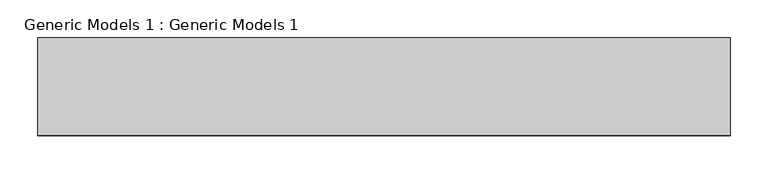
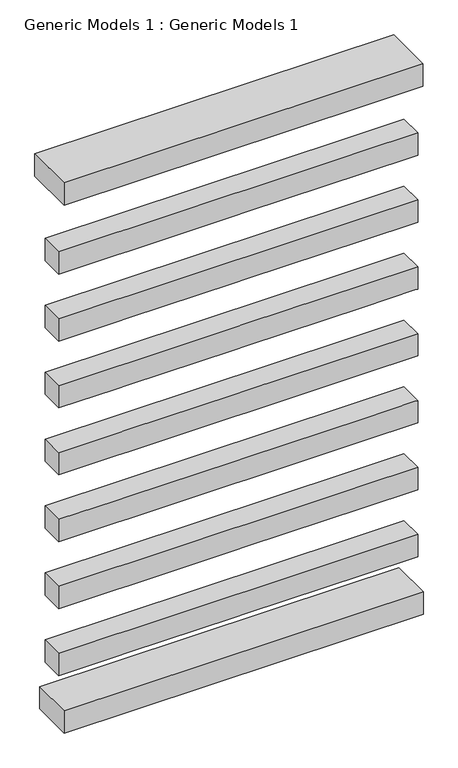
"""IFC4 building model written with IfcOpenShell, lengths in millimetres: proxy geometry, Generic Models 1 : Generic Models 1."""

from ifc_helpers import new_model, si_unit, origin, place, context, project, spatial, faceted_brep, source, transform, mapped, element, save


def generic_models_1_generic_models_1_5ca79dfd(model_context):
    return source(origin(), model_context, "Body", "Brep", [
        faceted_brep([(-2400.2544048, -6113.8685722, -385.6320944), (-2400.2544048, -6221.5933823, -385.6320944), (-2400.2544048, -6221.5933823, -445.6320944), (-2400.2544048, -6113.8685722, -445.6320944), (-3314.6544048, -6113.8685722, -385.6320944), (-3314.6544048, -6113.8685722, -445.6320944), (-3314.6544048, -6221.5933823, -445.6320944), (-3314.6544048, -6221.5933823, -385.6320944), (-2407.8544048, -6113.8685722, -385.6320944), (-2538.5868425, -6113.8685722, -385.6320944), (-2538.5868425, -6113.8685722, -445.6320944), (-2407.8544048, -6113.8685722, -445.6320944)], [[[0, 1, 2, 3]], [[4, 5, 6, 7]], [[1, 0, 8, 9, 4, 7]], [[2, 1, 7, 6]], [[3, 2, 6, 5, 10, 11]], [[0, 3, 11, 10, 5, 4, 9, 8]]]),
        faceted_brep([(-2400.2544048, -6137.2837816, -245.6320944), (-2400.2544048, -6197.2837816, -245.6320944), (-2400.2544048, -6197.2837816, -305.6320944), (-2400.2544048, -6137.2837816, -305.6320944), (-3314.6544048, -6137.2837816, -245.6320944), (-3314.6544048, -6137.2837816, -305.6320944), (-3314.6544048, -6197.2837816, -305.6320944), (-3314.6544048, -6197.2837816, -245.6320944), (-2407.8544048, -6137.2837816, -245.6320944), (-2538.5868425, -6137.2837816, -245.6320944), (-3169.36382, -6197.2837816, -245.6320944), (-3136.5029848, -6197.2837816, -245.6320944), (-2869.36382, -6197.2837816, -245.6320944), (-2836.5029848, -6197.2837816, -245.6320944), (-2538.5868425, -6197.2837816, -245.6320944), (-2407.8544048, -6197.2837816, -245.6320944), (-3169.36382, -6197.2837816, -305.6320944), (-3136.5029848, -6197.2837816, -305.6320944), (-2869.36382, -6197.2837816, -305.6320944), (-2836.5029848, -6197.2837816, -305.6320944), (-2538.5868425, -6197.2837816, -305.6320944), (-2407.8544048, -6197.2837816, -305.6320944), (-2538.5868425, -6137.2837816, -305.6320944), (-2407.8544048, -6137.2837816, -305.6320944)], [[[0, 1, 2, 3]], [[4, 5, 6, 7]], [[1, 0, 8, 9, 4, 7, 10, 11, 12, 13, 14, 15]], [[2, 1, 15, 14, 13, 12, 11, 10, 7, 6, 16, 17, 18, 19, 20, 21]], [[3, 2, 21, 20, 19, 18, 17, 16, 6, 5, 22, 23]], [[0, 3, 23, 22, 5, 4, 9, 8]]]),
        faceted_brep([(-2400.2544048, -6137.2837816, -65.6320944), (-2400.2544048, -6197.2837816, -65.6320944), (-2400.2544048, -6197.2837816, -125.6320944), (-2400.2544048, -6137.2837816, -125.6320944), (-3314.6544048, -6137.2837816, -65.6320944), (-3314.6544048, -6137.2837816, -125.6320944), (-3314.6544048, -6197.2837816, -125.6320944), (-3314.6544048, -6197.2837816, -65.6320944), (-2407.8544048, -6137.2837816, -65.6320944), (-2538.5868425, -6137.2837816, -65.6320944), (-3169.36382, -6197.2837816, -65.6320944), (-3136.5029848, -6197.2837816, -65.6320944), (-2869.36382, -6197.2837816, -65.6320944), (-2836.5029848, -6197.2837816, -65.6320944), (-2538.5868425, -6197.2837816, -65.6320944), (-2407.8544048, -6197.2837816, -65.6320944), (-3169.36382, -6197.2837816, -125.6320944), (-3136.5029848, -6197.2837816, -125.6320944), (-2869.36382, -6197.2837816, -125.6320944), (-2836.5029848, -6197.2837816, -125.6320944), (-2538.5868425, -6197.2837816, -125.6320944), (-2407.8544048, -6197.2837816, -125.6320944), (-2538.5868425, -6137.2837816, -125.6320944), (-2407.8544048, -6137.2837816, -125.6320944)], [[[0, 1, 2, 3]], [[4, 5, 6, 7]], [[1, 0, 8, 9, 4, 7, 10, 11, 12, 13, 14, 15]], [[2, 1, 15, 14, 13, 12, 11, 10, 7, 6, 16, 17, 18, 19, 20, 21]], [[3, 2, 21, 20, 19, 18, 17, 16, 6, 5, 22, 23]], [[0, 3, 23, 22, 5, 4, 9, 8]]]),
        faceted_brep([(-2400.2544048, -6137.2837816, 114.3679056), (-2400.2544048, -6197.2837816, 114.3679056), (-2400.2544048, -6197.2837816, 54.3679056), (-2400.2544048, -6137.2837816, 54.3679056), (-3314.6544048, -6137.2837816, 114.3679056), (-3314.6544048, -6137.2837816, 54.3679056), (-3314.6544048, -6197.2837816, 54.3679056), (-3314.6544048, -6197.2837816, 114.3679056), (-2407.8544048, -6137.2837816, 114.3679056), (-2538.5868425, -6137.2837816, 114.3679056), (-3169.36382, -6197.2837816, 114.3679056), (-3136.5029848, -6197.2837816, 114.3679056), (-2869.36382, -6197.2837816, 114.3679056), (-2836.5029848, -6197.2837816, 114.3679056), (-2538.5868425, -6197.2837816, 114.3679056), (-2407.8544048, -6197.2837816, 114.3679056), (-3169.36382, -6197.2837816, 54.3679056), (-3136.5029848, -6197.2837816, 54.3679056), (-2869.36382, -6197.2837816, 54.3679056), (-2836.5029848, -6197.2837816, 54.3679056), (-2538.5868425, -6197.2837816, 54.3679056), (-2407.8544048, -6197.2837816, 54.3679056), (-2538.5868425, -6137.2837816, 54.3679056), (-2407.8544048, -6137.2837816, 54.3679056)], [[[0, 1, 2, 3]], [[4, 5, 6, 7]], [[1, 0, 8, 9, 4, 7, 10, 11, 12, 13, 14, 15]], [[2, 1, 15, 14, 13, 12, 11, 10, 7, 6, 16, 17, 18, 19, 20, 21]], [[3, 2, 21, 20, 19, 18, 17, 16, 6, 5, 22, 23]], [[0, 3, 23, 22, 5, 4, 9, 8]]]),
        faceted_brep([(-2400.2544048, -6137.2837816, 294.3679056), (-2400.2544048, -6197.2837816, 294.3679056), (-2400.2544048, -6197.2837816, 234.3679056), (-2400.2544048, -6137.2837816, 234.3679056), (-3314.6544048, -6137.2837816, 294.3679056), (-3314.6544048, -6137.2837816, 234.3679056), (-3314.6544048, -6197.2837816, 234.3679056), (-3314.6544048, -6197.2837816, 294.3679056), (-2407.8544048, -6137.2837816, 294.3679056), (-2538.5868425, -6137.2837816, 294.3679056), (-3169.36382, -6197.2837816, 294.3679056), (-3136.5029848, -6197.2837816, 294.3679056), (-2869.36382, -6197.2837816, 294.3679056), (-2836.5029848, -6197.2837816, 294.3679056), (-2538.5868425, -6197.2837816, 294.3679056), (-2407.8544048, -6197.2837816, 294.3679056), (-3169.36382, -6197.2837816, 234.3679056), (-3136.5029848, -6197.2837816, 234.3679056), (-2869.36382, -6197.2837816, 234.3679056), (-2836.5029848, -6197.2837816, 234.3679056), (-2538.5868425, -6197.2837816, 234.3679056), (-2407.8544048, -6197.2837816, 234.3679056), (-2538.5868425, -6137.2837816, 234.3679056), (-2407.8544048, -6137.2837816, 234.3679056)], [[[0, 1, 2, 3]], [[4, 5, 6, 7]], [[1, 0, 8, 9, 4, 7, 10, 11, 12, 13, 14, 15]], [[2, 1, 15, 14, 13, 12, 11, 10, 7, 6, 16, 17, 18, 19, 20, 21]], [[3, 2, 21, 20, 19, 18, 17, 16, 6, 5, 22, 23]], [[0, 3, 23, 22, 5, 4, 9, 8]]]),
        faceted_brep([(-2400.2544048, -6137.2837816, 474.3679056), (-2400.2544048, -6197.2837816, 474.3679056), (-2400.2544048, -6197.2837816, 414.3679056), (-2400.2544048, -6137.2837816, 414.3679056), (-3314.6544048, -6137.2837816, 474.3679056), (-3314.6544048, -6137.2837816, 414.3679056), (-3314.6544048, -6197.2837816, 414.3679056), (-3314.6544048, -6197.2837816, 474.3679056), (-2407.8544048, -6137.2837816, 474.3679056), (-2538.5868425, -6137.2837816, 474.3679056), (-3169.36382, -6197.2837816, 474.3679056), (-3136.5029848, -6197.2837816, 474.3679056), (-2869.36382, -6197.2837816, 474.3679056), (-2836.5029848, -6197.2837816, 474.3679056), (-2538.5868425, -6197.2837816, 474.3679056), (-2407.8544048, -6197.2837816, 474.3679056), (-3169.36382, -6197.2837816, 414.3679056), (-3136.5029848, -6197.2837816, 414.3679056), (-2869.36382, -6197.2837816, 414.3679056), (-2836.5029848, -6197.2837816, 414.3679056), (-2538.5868425, -6197.2837816, 414.3679056), (-2407.8544048, -6197.2837816, 414.3679056), (-2538.5868425, -6137.2837816, 414.3679056), (-2407.8544048, -6137.2837816, 414.3679056)], [[[0, 1, 2, 3]], [[4, 5, 6, 7]], [[1, 0, 8, 9, 4, 7, 10, 11, 12, 13, 14, 15]], [[2, 1, 15, 14, 13, 12, 11, 10, 7, 6, 16, 17, 18, 19, 20, 21]], [[3, 2, 21, 20, 19, 18, 17, 16, 6, 5, 22, 23]], [[0, 3, 23, 22, 5, 4, 9, 8]]]),
        faceted_brep([(-2400.2544048, -6137.2837816, 654.3679056), (-2400.2544048, -6197.2837816, 654.3679056), (-2400.2544048, -6197.2837816, 594.3679056), (-2400.2544048, -6137.2837816, 594.3679056), (-3314.6544048, -6137.2837816, 654.3679056), (-3314.6544048, -6137.2837816, 594.3679056), (-3314.6544048, -6197.2837816, 594.3679056), (-3314.6544048, -6197.2837816, 654.3679056), (-2407.8544048, -6137.2837816, 654.3679056), (-2538.5868425, -6137.2837816, 654.3679056), (-3169.36382, -6197.2837816, 654.3679056), (-3136.5029848, -6197.2837816, 654.3679056), (-2869.36382, -6197.2837816, 654.3679056), (-2836.5029848, -6197.2837816, 654.3679056), (-2538.5868425, -6197.2837816, 654.3679056), (-2407.8544048, -6197.2837816, 654.3679056), (-3169.36382, -6197.2837816, 594.3679056), (-3136.5029848, -6197.2837816, 594.3679056), (-2869.36382, -6197.2837816, 594.3679056), (-2836.5029848, -6197.2837816, 594.3679056), (-2538.5868425, -6197.2837816, 594.3679056), (-2407.8544048, -6197.2837816, 594.3679056), (-2538.5868425, -6137.2837816, 594.3679056), (-2407.8544048, -6137.2837816, 594.3679056)], [[[0, 1, 2, 3]], [[4, 5, 6, 7]], [[1, 0, 8, 9, 4, 7, 10, 11, 12, 13, 14, 15]], [[2, 1, 15, 14, 13, 12, 11, 10, 7, 6, 16, 17, 18, 19, 20, 21]], [[3, 2, 21, 20, 19, 18, 17, 16, 6, 5, 22, 23]], [[0, 3, 23, 22, 5, 4, 9, 8]]]),
        faceted_brep([(-2400.2544048, -6137.2837816, 834.3679056), (-2400.2544048, -6197.2837816, 834.3679056), (-2400.2544048, -6197.2837816, 774.3679056), (-2400.2544048, -6137.2837816, 774.3679056), (-3314.6544048, -6137.2837816, 834.3679056), (-3314.6544048, -6137.2837816, 774.3679056), (-3314.6544048, -6197.2837816, 774.3679056), (-3314.6544048, -6197.2837816, 834.3679056), (-2407.8544048, -6137.2837816, 834.3679056), (-2538.5868425, -6137.2837816, 834.3679056), (-3169.36382, -6197.2837816, 834.3679056), (-3136.5029848, -6197.2837816, 834.3679056), (-2869.36382, -6197.2837816, 834.3679056), (-2836.5029848, -6197.2837816, 834.3679056), (-2538.5868425, -6197.2837816, 834.3679056), (-2407.8544048, -6197.2837816, 834.3679056), (-3169.36382, -6197.2837816, 774.3679056), (-3136.5029848, -6197.2837816, 774.3679056), (-2869.36382, -6197.2837816, 774.3679056), (-2836.5029848, -6197.2837816, 774.3679056), (-2538.5868425, -6197.2837816, 774.3679056), (-2407.8544048, -6197.2837816, 774.3679056), (-2538.5868425, -6137.2837816, 774.3679056), (-2407.8544048, -6137.2837816, 774.3679056)], [[[0, 1, 2, 3]], [[4, 5, 6, 7]], [[1, 0, 8, 9, 4, 7, 10, 11, 12, 13, 14, 15]], [[2, 1, 15, 14, 13, 12, 11, 10, 7, 6, 16, 17, 18, 19, 20, 21]], [[3, 2, 21, 20, 19, 18, 17, 16, 6, 5, 22, 23]], [[0, 3, 23, 22, 5, 4, 9, 8]]]),
        faceted_brep([(-2400.2544048, -6092.2648653, 1034.3679056), (-2400.2544048, -6220.9896754, 1034.3679056), (-2400.2544048, -6220.9896754, 974.3679056), (-2400.2544048, -6092.2648653, 974.3679056), (-3314.6544048, -6092.2648653, 1034.3679056), (-3314.6544048, -6092.2648653, 974.3679056), (-3314.6544048, -6220.9896754, 974.3679056), (-3314.6544048, -6220.9896754, 1034.3679056), (-2538.5868425, -6220.9896754, 974.3679056), (-2407.8544048, -6220.9896754, 974.3679056), (-2538.5868425, -6092.2648653, 974.3679056), (-2407.8544048, -6092.2648653, 974.3679056)], [[[0, 1, 2, 3]], [[4, 5, 6, 7]], [[1, 0, 4, 7]], [[2, 1, 7, 6, 8, 9]], [[3, 2, 9, 8, 6, 5, 10, 11]], [[0, 3, 11, 10, 5, 4]]]),
    ])


if __name__ == "__main__":
    model = new_model("IFC4")
    model_context = context("Model", 3, world=origin())
    ifc_project = project(units=[si_unit("LENGTHUNIT", "METRE", prefix="MILLI")], contexts=[model_context])
    site = spatial("IfcSite", under=ifc_project)
    building = spatial("IfcBuilding", under=site)
    placement = place(None, origin())
    generic_models_1_generic_models_1_shape = generic_models_1_generic_models_1_5ca79dfd(model_context)
    element("IfcBuildingElementProxy", 1, Name="Generic Models 1 : Generic Models 1", ObjectType="Generic Models 1 : Generic Models 1", at=placement, inside=building, context=model_context, shape_type="MappedRepresentation", body=[
        mapped(generic_models_1_generic_models_1_shape, transform((0.0, 0.0, 0.0), x_axis=(1.0, 0.0, 0.0), y_axis=(0.0, 1.0, 0.0), z_axis=(0.0, 0.0, 1.0))),
    ])
    save(model, "model.ifc")
